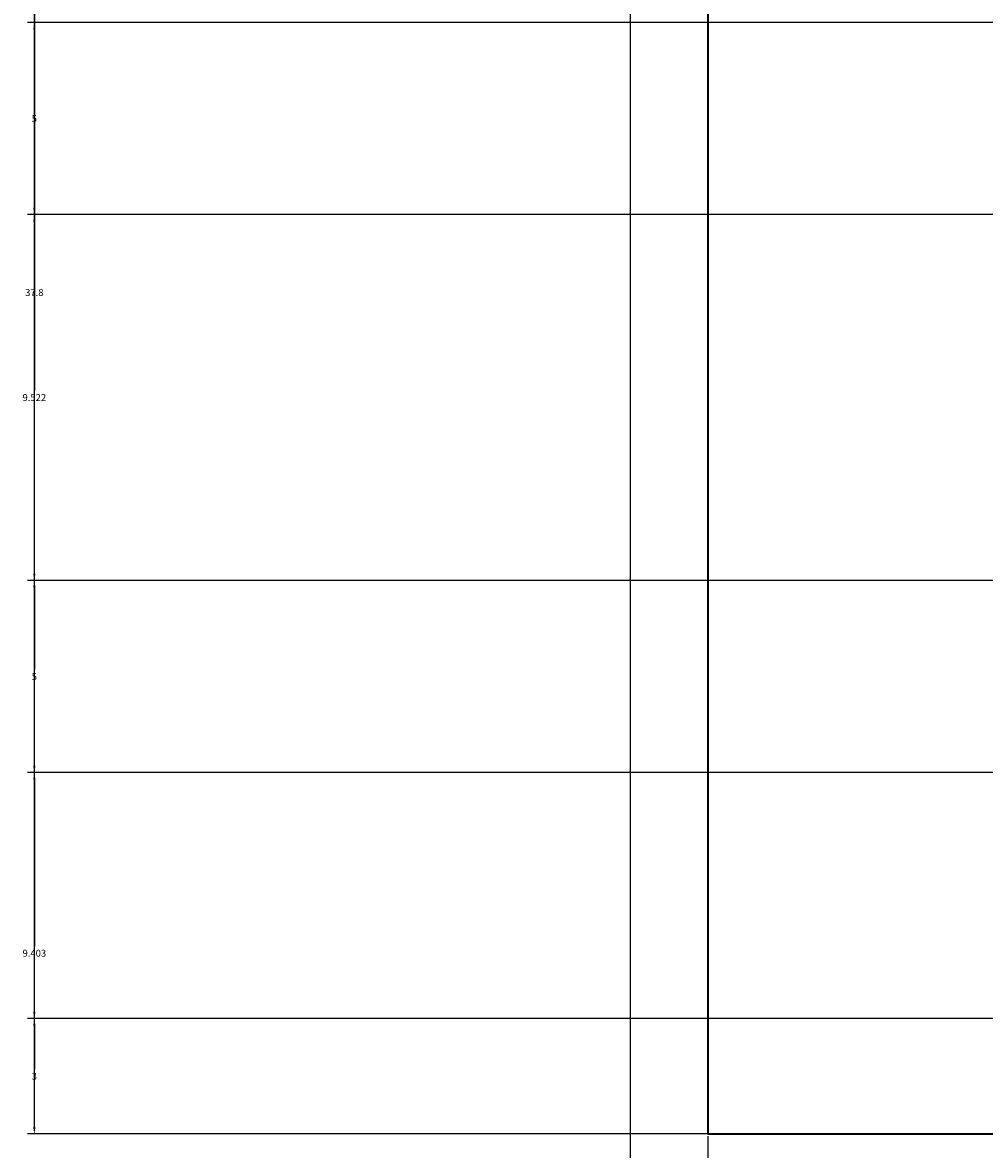
# Model space of a CAD drawing. Units: inches. Extents: x -6 to 289, y -8 to 323.
# Tile 2 of 107: x -6 to 19, y 7 to 36. Entities that reach past the tile are written whole.
import ezdxf

# ---------------------------------------------------------------- set-up
doc = ezdxf.new("R2010")
doc.units = ezdxf.units.IN
doc.header["$MEASUREMENT"] = 0
doc.layers.add('A-ANNO-DIMS', color=2, linetype='Continuous', lineweight=18)
doc.layers.add('A-ELEV', color=7, linetype='Continuous', lineweight=35)
doc.styles.get("Standard").update_dxf_attribs({"font": 'arial.ttf'})
doc.dimstyles.get("Standard").update_dxf_attribs({"dimtxt": 0.18, "dimasz": 0.18, "dimexe": 0.18, "dimexo": 0.0625, "dimgap": 0.09, "dimtad": 0, "dimtih": 1, "dimtoh": 1, "dimdec": 4, "dimzin": 0, "dimdsep": 46, "dimtxsty": 'Standard', "dimcen": 0.09, "dimadec": 0, "dimazin": 0, "dimtfac": 1, "dimtdec": 4, "dimtofl": 0, "dimtmove": 0, "dimatfit": 3, "dimfxl": 1, "dimtolj": 1, "dimtzin": 0, "dimarcsym": 0})

# ---------------------------------------------------------------- blocks, each defined once
blk = doc.blocks.new('*D16')
at = {"layer": 'A-ANNO-DIMS', "color": 0, "lineweight": -2, "transparency": 16777216}
for p, q in [((9.943, 68.37), (9.943, -8.391)), ((272.973, 68.37), (272.973, -8.391)), ((10.123, -8.211), (140.993, -8.211)), ((272.793, -8.211), (141.923, -8.211))]:
    blk.add_line(p, q, dxfattribs=at)
at = {"layer": 'A-ANNO-DIMS', "color": 0, "transparency": 16777216}
for points in [[(10.123, -8.181), (10.123, -8.241), (9.943, -8.211)], [(272.793, -8.181), (272.793, -8.241), (272.973, -8.211)]]:
    blk.add_solid(points, dxfattribs=at)
at = {"layer": 'Defpoints', "color": 0, "transparency": 16777216}
for p in [(9.943, 68.432), (272.973, 68.432), (272.973, -8.211)]:
    blk.add_point(p, dxfattribs=at)
at = {"layer": 'A-ANNO-DIMS', "color": 0, "transparency": 16777216, "insert": (141.458, -8.211), "char_height": 0.18, "attachment_point": 5}
blk.add_mtext('\\A1;263.03', dxfattribs=at)
blk = doc.blocks.new('*D17')
at = {"layer": 'A-ANNO-DIMS', "color": 0, "lineweight": -2, "transparency": 16777216}
for p, q in [((33.681, 70.243), (-5.737, 70.243)), ((-5.557, 70.063), (-5.557, 38.948)), ((-5.557, 7.469), (-5.557, 38.584)), ((11.907, 7.289), (-5.737, 7.289))]:
    blk.add_line(p, q, dxfattribs=at)
at = {"layer": 'A-ANNO-DIMS', "color": 0, "transparency": 16777216}
for points in [[(-5.587, 70.063), (-5.527, 70.063), (-5.557, 70.243)], [(-5.587, 7.469), (-5.527, 7.469), (-5.557, 7.289)]]:
    blk.add_solid(points, dxfattribs=at)
at = {"layer": 'Defpoints', "color": 0, "transparency": 16777216}
for p in [(-5.557, 70.243), (33.744, 70.243), (11.969, 7.289)]:
    blk.add_point(p, dxfattribs=at)
at = {"layer": 'A-ANNO-DIMS', "color": 0, "transparency": 16777216, "insert": (-5.557, 38.766), "char_height": 0.18, "attachment_point": 5}
blk.add_mtext('\\A1;62.95', dxfattribs=at)
blk = doc.blocks.new('*D22')
at = {"layer": 'A-ANNO-DIMS', "color": 0, "lineweight": -2, "transparency": 16777216}
for p, q in [((19.101, 307.289), (-5.737, 307.289)), ((-5.557, 307.109), (-5.557, 157.471)), ((-5.557, 7.469), (-5.557, 157.107)), ((11.907, 7.289), (-5.737, 7.289))]:
    blk.add_line(p, q, dxfattribs=at)
at = {"layer": 'A-ANNO-DIMS', "color": 0, "transparency": 16777216}
for points in [[(-5.587, 307.109), (-5.527, 307.109), (-5.557, 307.289)], [(-5.587, 7.469), (-5.527, 7.469), (-5.557, 7.289)]]:
    blk.add_solid(points, dxfattribs=at)
at = {"layer": 'Defpoints', "color": 0, "transparency": 16777216}
for p in [(19.164, 307.289), (-5.557, 7.289), (11.969, 7.289)]:
    blk.add_point(p, dxfattribs=at)
at = {"layer": 'A-ANNO-DIMS', "color": 0, "transparency": 16777216, "insert": (-5.557, 157.289), "char_height": 0.18, "attachment_point": 5}
blk.add_mtext('\\A1;300', dxfattribs=at)
blk = doc.blocks.new('*D50')
at = {"layer": 'A-ANNO-DIMS', "color": 0, "lineweight": -2, "transparency": 16777216}
for p, q in [((11.969, 7.226), (11.969, -8.391)), ((24.317, 7.226), (24.317, -8.391)), ((12.149, -8.211), (17.688, -8.211)), ((24.137, -8.211), (18.598, -8.211))]:
    blk.add_line(p, q, dxfattribs=at)
at = {"layer": 'A-ANNO-DIMS', "color": 0, "transparency": 16777216}
for points in [[(12.149, -8.181), (12.149, -8.241), (11.969, -8.211)], [(24.137, -8.181), (24.137, -8.241), (24.317, -8.211)]]:
    blk.add_solid(points, dxfattribs=at)
at = {"layer": 'Defpoints', "color": 0, "transparency": 16777216}
for p in [(11.969, 7.289), (24.317, 7.289), (24.317, -8.211)]:
    blk.add_point(p, dxfattribs=at)
at = {"layer": 'A-ANNO-DIMS', "color": 0, "transparency": 16777216, "insert": (18.143, -8.211), "char_height": 0.18, "attachment_point": 5}
blk.add_mtext('\\A1;12.348', dxfattribs=at)
blk = doc.blocks.new('*D59')
at = {"layer": 'A-ANNO-DIMS', "color": 0, "lineweight": -2, "transparency": 16777216}
for p, q in [((39.647, 16.692), (-5.737, 16.692)), ((-5.557, 16.512), (-5.557, 12.172)), ((-5.557, 7.469), (-5.557, 11.808)), ((11.907, 7.289), (-5.737, 7.289))]:
    blk.add_line(p, q, dxfattribs=at)
at = {"layer": 'A-ANNO-DIMS', "color": 0, "transparency": 16777216}
for points in [[(-5.587, 16.512), (-5.527, 16.512), (-5.557, 16.692)], [(-5.587, 7.469), (-5.527, 7.469), (-5.557, 7.289)]]:
    blk.add_solid(points, dxfattribs=at)
at = {"layer": 'Defpoints', "color": 0, "transparency": 16777216}
for p in [(-5.557, 16.692), (39.709, 16.692), (11.969, 7.289)]:
    blk.add_point(p, dxfattribs=at)
at = {"layer": 'A-ANNO-DIMS', "color": 0, "transparency": 16777216, "insert": (-5.557, 11.99), "char_height": 0.18, "attachment_point": 5}
blk.add_mtext('\\A1;9.403', dxfattribs=at)
blk = doc.blocks.new('*D60')
at = {"layer": 'A-ANNO-DIMS', "color": 0, "lineweight": -2, "transparency": 16777216}
for p, q in [((44.647, 21.692), (-5.737, 21.692)), ((-5.557, 21.512), (-5.557, 19.373)), ((-5.557, 16.872), (-5.557, 19.01)), ((39.647, 16.692), (-5.737, 16.692))]:
    blk.add_line(p, q, dxfattribs=at)
at = {"layer": 'A-ANNO-DIMS', "color": 0, "transparency": 16777216}
for points in [[(-5.587, 21.512), (-5.527, 21.512), (-5.557, 21.692)], [(-5.587, 16.872), (-5.527, 16.872), (-5.557, 16.692)]]:
    blk.add_solid(points, dxfattribs=at)
at = {"layer": 'Defpoints', "color": 0, "transparency": 16777216}
for p in [(-5.557, 21.692), (44.709, 21.692), (39.709, 16.692)]:
    blk.add_point(p, dxfattribs=at)
at = {"layer": 'A-ANNO-DIMS', "color": 0, "transparency": 16777216, "insert": (-5.557, 19.192), "char_height": 0.18, "attachment_point": 5}
blk.add_mtext('\\A1;5', dxfattribs=at)
blk = doc.blocks.new('*D61')
at = {"layer": 'A-ANNO-DIMS', "color": 0, "lineweight": -2, "transparency": 16777216}
for p, q in [((44.647, 31.213), (-5.737, 31.213)), ((-5.557, 31.033), (-5.557, 26.634)), ((-5.557, 21.872), (-5.557, 26.271)), ((44.647, 21.692), (-5.737, 21.692))]:
    blk.add_line(p, q, dxfattribs=at)
at = {"layer": 'A-ANNO-DIMS', "color": 0, "transparency": 16777216}
for points in [[(-5.587, 31.033), (-5.527, 31.033), (-5.557, 31.213)], [(-5.587, 21.872), (-5.527, 21.872), (-5.557, 21.692)]]:
    blk.add_solid(points, dxfattribs=at)
at = {"layer": 'Defpoints', "color": 0, "transparency": 16777216}
for p in [(-5.557, 31.213), (44.709, 31.213), (44.709, 21.692)]:
    blk.add_point(p, dxfattribs=at)
at = {"layer": 'A-ANNO-DIMS', "color": 0, "transparency": 16777216, "insert": (-5.557, 26.453), "char_height": 0.18, "attachment_point": 5}
blk.add_mtext('\\A1;9.522', dxfattribs=at)
blk = doc.blocks.new('*D62')
at = {"layer": 'A-ANNO-DIMS', "color": 0, "lineweight": -2, "transparency": 16777216}
for p, q in [((39.647, 36.213), (-5.737, 36.213)), ((-5.557, 36.033), (-5.557, 33.895)), ((-5.557, 31.393), (-5.557, 33.532)), ((44.647, 31.213), (-5.737, 31.213))]:
    blk.add_line(p, q, dxfattribs=at)
at = {"layer": 'A-ANNO-DIMS', "color": 0, "transparency": 16777216}
for points in [[(-5.587, 36.033), (-5.527, 36.033), (-5.557, 36.213)], [(-5.587, 31.393), (-5.527, 31.393), (-5.557, 31.213)]]:
    blk.add_solid(points, dxfattribs=at)
at = {"layer": 'Defpoints', "color": 0, "transparency": 16777216}
for p in [(-5.557, 36.213), (39.709, 36.213), (44.709, 31.213)]:
    blk.add_point(p, dxfattribs=at)
at = {"layer": 'A-ANNO-DIMS', "color": 0, "transparency": 16777216, "insert": (-5.557, 33.713), "char_height": 0.18, "attachment_point": 5}
blk.add_mtext('\\A1;5', dxfattribs=at)
blk = doc.blocks.new('*D83')
at = {"layer": 'A-ANNO-DIMS', "color": 0, "lineweight": -2, "transparency": 16777216}
for p, q in [((123.945, 10.289), (-5.737, 10.289)), ((-5.557, 10.109), (-5.557, 8.971)), ((-5.557, 7.469), (-5.557, 8.607)), ((120.945, 7.289), (-5.737, 7.289))]:
    blk.add_line(p, q, dxfattribs=at)
at = {"layer": 'A-ANNO-DIMS', "color": 0, "transparency": 16777216}
for points in [[(-5.587, 10.109), (-5.527, 10.109), (-5.557, 10.289)], [(-5.587, 7.469), (-5.527, 7.469), (-5.557, 7.289)]]:
    blk.add_solid(points, dxfattribs=at)
at = {"layer": 'Defpoints', "color": 0, "transparency": 16777216}
for p in [(-5.557, 10.289), (124.008, 10.289), (121.008, 7.289)]:
    blk.add_point(p, dxfattribs=at)
at = {"layer": 'A-ANNO-DIMS', "color": 0, "transparency": 16777216, "insert": (-5.557, 8.789), "char_height": 0.18, "attachment_point": 5}
blk.add_mtext('\\A1;3', dxfattribs=at)
blk = doc.blocks.new('*D84')
at = {"layer": 'A-ANNO-DIMS', "color": 0, "lineweight": -2, "transparency": 16777216}
for p, q in [((123.945, 48.085), (-5.737, 48.085)), ((-5.557, 47.905), (-5.557, 29.369)), ((-5.557, 10.469), (-5.557, 29.005)), ((123.945, 10.289), (-5.737, 10.289))]:
    blk.add_line(p, q, dxfattribs=at)
at = {"layer": 'A-ANNO-DIMS', "color": 0, "transparency": 16777216}
for points in [[(-5.587, 47.905), (-5.527, 47.905), (-5.557, 48.085)], [(-5.587, 10.469), (-5.527, 10.469), (-5.557, 10.289)]]:
    blk.add_solid(points, dxfattribs=at)
at = {"layer": 'Defpoints', "color": 0, "transparency": 16777216}
for p in [(-5.557, 48.085), (124.008, 48.085), (124.008, 10.289)]:
    blk.add_point(p, dxfattribs=at)
at = {"layer": 'A-ANNO-DIMS', "color": 0, "transparency": 16777216, "insert": (-5.557, 29.187), "char_height": 0.18, "attachment_point": 5}
blk.add_mtext('\\A1;37.8', dxfattribs=at)

msp = doc.modelspace()

# ---------------------------------------------------------------- linework, layer by layer
at = {"layer": 'A-ELEV'}
msp.add_lwpolyline([(11.9692, 66.2238), (11.9692, 7.2888), (24.317, 7.2888), (24.317, 66.2238)], dxfattribs=at)

# ---------------------------------------------------------------- dimensions: what is measured, and where the dimension line sits
at = {"layer": 'A-ANNO-DIMS'}
for base, p1, p2, override, picture, middle in [((-5.557, 7.2888), (19.1638, 307.2888), (11.9692, 7.2888), {"dimdec": 0, "dimlfac": 1, "dimrnd": 0, "dimzin": 0, "dimdsep": 46, "dimlunit": 2}, '*D22', (-5.557, 157.2888)), ((-5.557, 70.2425), (11.9692, 7.2888), (33.7437, 70.2425), {"dimdec": 2, "dimlfac": 1, "dimrnd": 0, "dimzin": 0, "dimdsep": 46, "dimlunit": 2}, '*D17', (-5.557, 38.7657)), ((-5.557, 48.0851), (124.008, 10.2888), (124.008, 48.0851), {"dimdec": 1, "dimlfac": 1, "dimrnd": 0, "dimzin": 0, "dimdsep": 46, "dimlunit": 2}, '*D84', (-5.557, 29.187)), ((-5.557, 36.2133), (44.709, 31.2133), (39.709, 36.2133), {"dimdec": 0, "dimlfac": 1, "dimrnd": 0, "dimzin": 0, "dimdsep": 46, "dimlunit": 2}, '*D62', (-5.557, 33.7133)), ((-5.557, 31.2133), (44.709, 21.6917), (44.709, 31.2133), {"dimdec": 3, "dimlfac": 1, "dimrnd": 0, "dimzin": 0, "dimdsep": 46, "dimlunit": 2}, '*D61', (-5.557, 26.4525)), ((-5.557, 21.6917), (39.709, 16.6917), (44.709, 21.6917), {"dimdec": 0, "dimlfac": 1, "dimrnd": 0, "dimzin": 0, "dimdsep": 46, "dimlunit": 2}, '*D60', (-5.557, 19.1917)), ((-5.557, 16.6917), (11.9692, 7.2888), (39.709, 16.6917), {"dimdec": 3, "dimlfac": 1, "dimrnd": 0, "dimzin": 0, "dimdsep": 46, "dimlunit": 2}, '*D59', (-5.557, 11.9902)), ((-5.557, 10.2888), (121.008, 7.2888), (124.008, 10.2888), {"dimdec": 0, "dimlfac": 1, "dimrnd": 0, "dimzin": 0, "dimdsep": 46, "dimlunit": 2}, '*D83', (-5.557, 8.7888))]:
    dim = msp.add_linear_dim(base=base, p1=p1, p2=p2, angle=90, dimstyle='Standard', override=override, dxfattribs=at)
    dim.commit()
    dim.dimension.update_dxf_attribs({"geometry": picture, "text_midpoint": middle})
for base, p1, p2, override, picture, middle in [((272.9733, -8.2112), (9.943, 68.4322), (272.9733, 68.4322), {"dimdec": 2, "dimlfac": 1, "dimrnd": 0, "dimzin": 0, "dimdsep": 46, "dimlunit": 2}, '*D16', (141.4581, -8.2112)), ((24.317, -8.2112), (11.9692, 7.2888), (24.317, 7.2888), {"dimdec": 3, "dimlfac": 1, "dimrnd": 0, "dimzin": 0, "dimdsep": 46, "dimlunit": 2}, '*D50', (18.1431, -8.2112))]:
    dim = msp.add_linear_dim(base=base, p1=p1, p2=p2, dimstyle='Standard', override=override, dxfattribs=at)
    dim.commit()
    dim.dimension.update_dxf_attribs({"geometry": picture, "text_midpoint": middle})

doc.saveas('drawing.dxf')
